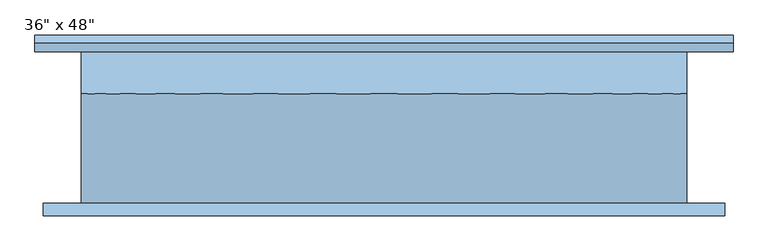
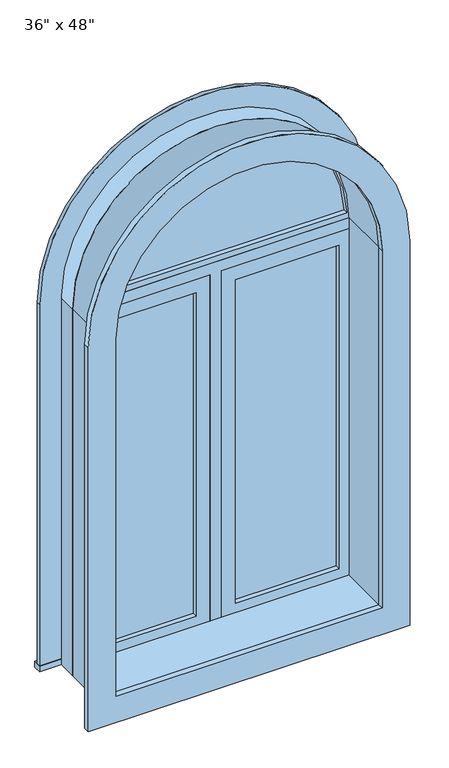
"""IFC4 building model written with IfcOpenShell, lengths in millimetres: window geometry."""

from ifc_helpers import new_model, si_unit, point, frame, frame_2d, origin, place, context, project, spatial, polyline, circle_curve, trimmed, segment, composite_curve, outline, extrude, source, transform, mapped, element, save


def window_ae0d0e3f(model_context):
    return source(origin(), model_context, "Body", "SweptSolid", [
        extrude(outline(composite_curve([segment(polyline([(1543.05, -506.3478419), (247.65, -506.3478419), (247.65, 522.3521581), (1543.05, 522.3521581)]), True, "CONTINUOUS"), segment(trimmed(circle_curve(frame_2d((1543.05, 8.0021581)), 514.35), [point((1543.05, 522.3521581))], [point((1543.05, -506.3478419))], False, "CARTESIAN"), True, "CONTINUOUS")], self_intersect=False), holes=[composite_curve([segment(trimmed(circle_curve(frame_2d((1543.05, 8.0021581)), 425.45), [point((1543.05, -417.4478419))], [point((1543.05, 433.4521581))], True, "CARTESIAN"), True, "CONTINUOUS"), segment(polyline([(1543.05, 433.4521581), (336.55, 433.4521581), (336.55, -417.4478419), (1543.05, -417.4478419)]), True, "CONTINUOUS")], self_intersect=False)]), frame((0.0, -133.35, 0.0), z_axis=(0.0, 1.0, 0.0), x_axis=(0.0, 0.0, 1.0)), (0.0, 0.0, 1.0), 19.05),
        extrude(outline(composite_curve([segment(trimmed(circle_curve(frame_2d((1543.05, 8.0021581)), 419.2154707), [point((1562.0999995, 426.7845699))], [point((1562.0999995, -410.7802537))], False, "CARTESIAN"), True, "CONTINUOUS"), segment(polyline([(1562.0999995, -410.7802537), (1562.0999995, 426.7845699)]), True, "CONTINUOUS")], self_intersect=False)), frame((0.0, 66.675, 0.0), z_axis=(0.0, 1.0, 0.0), x_axis=(0.0, 0.0, 1.0)), (0.0, 0.0, 1.0), 12.7),
        extrude(outline(composite_curve([segment(trimmed(circle_curve(frame_2d((1543.05, 8.0021581)), 438.15), [point((1543.05, 446.1521581))], [point((1543.05, -430.1478419))], False, "CARTESIAN"), True, "CONTINUOUS"), segment(polyline([(1543.05, -430.1478419), (1543.05, 446.1521581)]), True, "CONTINUOUS")], self_intersect=False), holes=[composite_curve([segment(polyline([(1562.0999995, 426.7845698), (1562.0999995, -410.7802537)]), True, "CONTINUOUS"), segment(trimmed(circle_curve(frame_2d((1543.05, 8.0021581)), 419.2154707), [point((1562.0999995, -410.7802537))], [point((1562.0999995, 426.7845698))], True, "CARTESIAN"), True, "CONTINUOUS")], self_intersect=False)]), frame((0.0, 50.8, 0.0), z_axis=(0.0, 1.0, 0.0), x_axis=(0.0, 0.0, 1.0)), (0.0, 0.0, 1.0), 44.45),
        extrude(outline(composite_curve([segment(polyline([(304.8, -449.1978419), (304.8, 465.2021581), (1543.05, 465.2021581)]), True, "CONTINUOUS"), segment(trimmed(circle_curve(frame_2d((1543.05, 8.0021581)), 457.2), [point((1543.05, 465.2021581))], [point((1543.05, -449.1978419))], False, "CARTESIAN"), True, "CONTINUOUS"), segment(polyline([(1543.05, -449.1978419), (304.8, -449.1978419)]), True, "CONTINUOUS")], self_intersect=False), holes=[composite_curve([segment(polyline([(323.85, -430.1478419), (1543.05, -430.1478419)]), True, "CONTINUOUS"), segment(trimmed(circle_curve(frame_2d((1543.05, 8.0021581)), 438.15), [point((1543.05, -430.1478419))], [point((1543.05, 446.1521581))], True, "CARTESIAN"), True, "CONTINUOUS"), segment(polyline([(1543.05, 446.1521581), (323.85, 446.1521581), (323.85, -430.1478419)]), True, "CONTINUOUS")], self_intersect=False)]), frame((0.0, 50.8, 0.0), z_axis=(0.0, 1.0, 0.0), x_axis=(0.0, 0.0, 1.0)), (0.0, 0.0, 1.0), 63.5),
        extrude(outline(polyline([(71.5021581, 79.375), (401.7021581, 79.375), (401.7021581, 66.675), (71.5021581, 66.675), (71.5021581, 79.375)])), frame((0.0, 0.0, 368.3), z_axis=(0.0, 0.0, 1.0), x_axis=(1.0, 0.0, 0.0)), (0.0, 0.0, 1.0), 1092.2),
        extrude(outline(polyline([(1504.95, 27.0521581), (323.85, 27.0521581), (323.85, 446.1521581), (1504.95, 446.1521581), (1504.95, 27.0521581)]), holes=[polyline([(1460.5, 71.5021581), (1460.5, 401.7021581), (368.3, 401.7021581), (368.3, 71.5021581), (1460.5, 71.5021581)])]), frame((0.0, 50.8, 0.0), z_axis=(0.0, 1.0, 0.0), x_axis=(0.0, 0.0, 1.0)), (0.0, 0.0, 1.0), 44.45),
        extrude(outline(polyline([(323.85, -11.0478419), (323.85, 27.0521581), (1504.95, 27.0521581), (1504.95, 446.1521581), (1543.05, 446.1521581), (1543.05, -430.1478419), (1504.95, -430.1478419), (1504.95, -11.0478419), (323.85, -11.0478419)])), frame((0.0, 50.8, 0.0), z_axis=(0.0, 1.0, 0.0), x_axis=(0.0, 0.0, 1.0)), (0.0, 0.0, 1.0), 63.5),
        extrude(outline(polyline([(-519.0478419, 139.7), (535.0521581, 139.7), (535.0521581, 114.3), (-519.0478419, 114.3), (-519.0478419, 139.7)])), frame((0.0, 0.0, 304.8), z_axis=(0.0, 0.0, 1.0), x_axis=(1.0, 0.0, 0.0)), (0.0, 0.0, 1.0), 19.05),
        extrude(outline(composite_curve([segment(polyline([(323.85, 446.1521581), (323.85, 535.0521581), (1543.05, 535.0521581)]), True, "CONTINUOUS"), segment(trimmed(circle_curve(frame_2d((1543.05, 8.0021581)), 527.05), [point((1543.05, 535.0521581))], [point((1543.05, -519.0478419))], False, "CARTESIAN"), True, "CONTINUOUS"), segment(polyline([(1543.05, -519.0478419), (323.85, -519.0478419), (323.85, -430.1478419), (1543.05, -430.1478419)]), True, "CONTINUOUS"), segment(trimmed(circle_curve(frame_2d((1543.05, 8.0021581)), 438.15), [point((1543.05, -430.1478419))], [point((1543.05, 446.1521581))], True, "CARTESIAN"), True, "CONTINUOUS"), segment(polyline([(1543.05, 446.1521581), (323.85, 446.1521581)]), True, "CONTINUOUS")], self_intersect=False)), frame((0.0, 114.3, 0.0), z_axis=(0.0, 1.0, 0.0), x_axis=(0.0, 0.0, 1.0)), (0.0, 0.0, 1.0), 12.7),
        extrude(outline(polyline([(-55.4978419, 66.675), (-385.6978419, 66.675), (-385.6978419, 79.375), (-55.4978419, 79.375), (-55.4978419, 66.675)])), frame((0.0, 0.0, 368.3), z_axis=(0.0, 0.0, 1.0), x_axis=(1.0, 0.0, 0.0)), (0.0, 0.0, 1.0), 1092.2),
        extrude(outline(polyline([(1504.95, -430.1478419), (323.85, -430.1478419), (323.85, -11.0478419), (1504.95, -11.0478419), (1504.95, -430.1478419)]), holes=[polyline([(1460.5, -385.6978419), (1460.5, -55.4978419), (368.3, -55.4978419), (368.3, -385.6978419), (1460.5, -385.6978419)])]), frame((0.0, 50.8, 0.0), z_axis=(0.0, 1.0, 0.0), x_axis=(0.0, 0.0, 1.0)), (0.0, 0.0, 1.0), 44.45),
        extrude(outline(composite_curve([segment(polyline([(304.8, 465.2021581), (1543.05, 465.2021581)]), True, "CONTINUOUS"), segment(trimmed(circle_curve(frame_2d((1543.05, 8.0021581)), 457.2), [point((1543.05, 465.2021581))], [point((1543.05, -449.1978419))], False, "CARTESIAN"), True, "CONTINUOUS"), segment(polyline([(1543.05, -449.1978419), (304.8, -449.1978419), (304.8, 465.2021581)]), True, "CONTINUOUS")], self_intersect=False), holes=[composite_curve([segment(polyline([(336.55, 433.4521581), (336.55, -417.4478419), (1543.05, -417.4478419)]), True, "CONTINUOUS"), segment(trimmed(circle_curve(frame_2d((1543.05, 8.0021581)), 425.45), [point((1543.05, -417.4478419))], [point((1543.05, 433.4521581))], True, "CARTESIAN"), True, "CONTINUOUS"), segment(polyline([(1543.05, 433.4521581), (336.55, 433.4521581)]), True, "CONTINUOUS")], self_intersect=False)]), frame((0.0, -114.3, 0.0), z_axis=(0.0, 1.0, 0.0), x_axis=(0.0, 0.0, 1.0)), (0.0, 0.0, 1.0), 165.1),
    ])


if __name__ == "__main__":
    model = new_model("IFC4")
    model_context = context("Model", 3, world=origin())
    ifc_project = project(units=[si_unit("LENGTHUNIT", "METRE", prefix="MILLI")], contexts=[model_context])
    site = spatial("IfcSite", under=ifc_project)
    building = spatial("IfcBuilding", under=site)
    placement = place(None, origin())
    window_shape = window_ae0d0e3f(model_context)
    element("IfcWindow", 1, ObjectType="36\" x 48\"", at=placement, inside=building, context=model_context, shape_type="MappedRepresentation", body=[
        mapped(window_shape, transform((0.0, 0.0, 0.0), x_axis=(1.0, 0.0, 0.0), y_axis=(0.0, 1.0, 0.0), z_axis=(0.0, 0.0, 1.0))),
    ])
    save(model, "model.ifc")

# Revit data of these elements
# Type "36\" x 48\""
#   Type Mark = "16"
#   Construction Type Id = "SGL"
#   Assembly Code = "B2020100"
#   Analytic Construction = "Large single-glazed windows"
#   Visual Light Transmittance = 0.9
#   Solar Heat Gain Coefficient = 0.86
#   Heat Transfer Coefficient (U) = 0.979472 BTU/(h·ft²·°F)
#   Height = 4' - 0"
#   Default Sill Height = 1' - 0"
#   Trim Projection - Ext. = 0' - 0 1/2"
#   Trim Projection - Int. = 0' - 0 3/4"
#   Trim Width - Exterior = 0' - 3 1/2"
#   Trim Width - Interior = 0' - 3 1/2"
#   Width = 3' - 0"
#   Window Inset = 0' - 0 3/4"
#   Define Thermal Properties by = 1
#   Glass Pane Material = Glass
#   Sash Material = Sash
#   Trim Exterior Material = Trim
#   Trim Interior Material = Trim
#   Wall Closure = (empty or 0)
# Element 1 (IfcWindow, "36\" x 48\"")
#   Materials on its faces: "Sash", "Trim", "Glass"
# Materials
#   "Glass": class "Glass", colour RGB 0 128 192, transparency 0.75, Description = "Soda Lime Glass", Cost = 0
#   "Sash": class "Wood", colour RGB 224 178 126, transparency 0
#   "Trim": class "Wood", colour RGB 224 178 126, transparency 0
